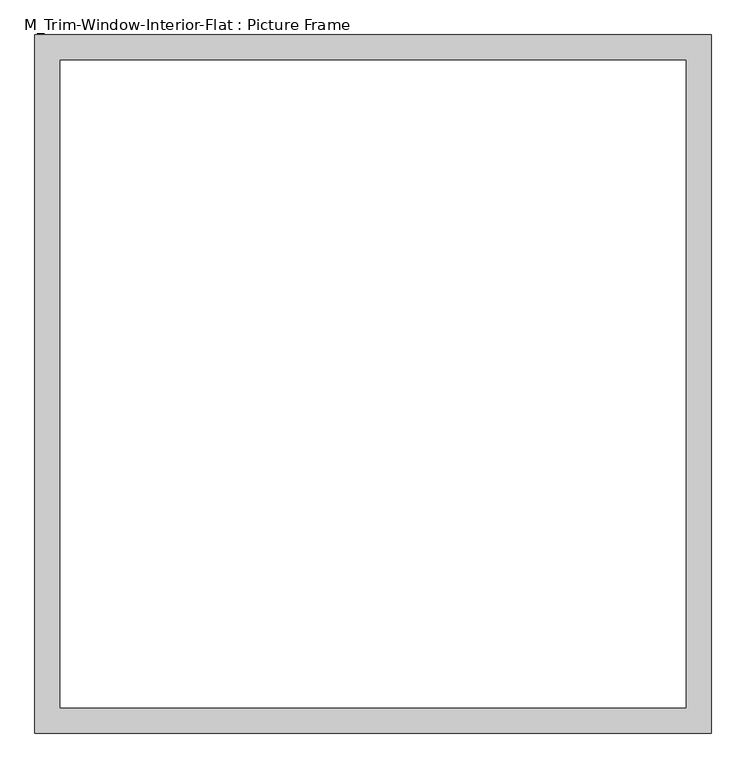
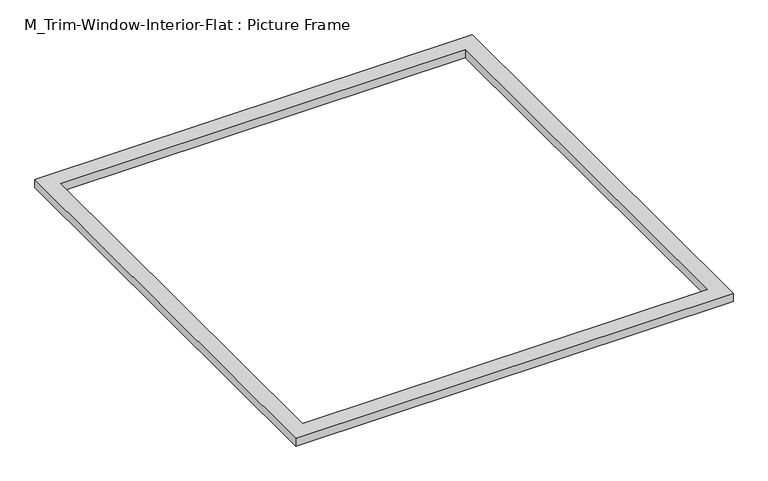
"""IFC4 building model written with IfcOpenShell, lengths in millimetres: proxy geometry, M_Trim-Window-Interior-Flat : Picture Frame."""

from ifc_helpers import new_model, si_unit, origin, origin_with_axes, place, context, project, spatial, polyline, outline, extrude, source, transform, mapped, element, save


def m_trim_window_interior_flat_picture_frame_44e8afef(model_context):
    return source(origin(), model_context, "Body", "SweptSolid", [
        extrude(outline(polyline([(797.3, 47.3), (797.3, -1598.1), (-797.3, -1598.1), (-797.3, 47.3), (797.3, 47.3)]), holes=[polyline([(737.3, -12.7), (-737.3, -12.7), (-737.3, -1538.1), (737.3, -1538.1), (737.3, -12.7)])]), origin_with_axes(), (0.0, 0.0, 1.0), 30.0),
    ])


if __name__ == "__main__":
    model = new_model("IFC4")
    model_context = context("Model", 3, world=origin())
    ifc_project = project(units=[si_unit("LENGTHUNIT", "METRE", prefix="MILLI")], contexts=[model_context])
    site = spatial("IfcSite", under=ifc_project)
    building = spatial("IfcBuilding", under=site)
    placement = place(None, origin())
    m_trim_window_interior_flat_picture_frame_shape = m_trim_window_interior_flat_picture_frame_44e8afef(model_context)
    element("IfcBuildingElementProxy", 1, Name="M_Trim-Window-Interior-Flat : Picture Frame", ObjectType="M_Trim-Window-Interior-Flat : Picture Frame", at=placement, inside=building, context=model_context, shape_type="MappedRepresentation", body=[
        mapped(m_trim_window_interior_flat_picture_frame_shape, transform((0.0, 0.0, 0.0), x_axis=(1.0, 0.0, 0.0), y_axis=(0.0, 1.0, 0.0), z_axis=(0.0, 0.0, 1.0))),
    ])
    save(model, "model.ifc")

# Revit data of these elements
# Type "M_Trim-Window-Interior-Flat : Picture Frame"
#   Trim Thickness_Picture Frame = 0' - 1.1811"
#   Trim Width = 0' - 2.3622"
#   Trim Thickness_with Sill = 0' - 0.7874"
#   Sill Thickness = 0' - 1.1811"
#   Opening Width [instance default] = 1' - 11.62205"
#   Opening Height [instance default] = 2' - 11.43307"
#   Default Elevation = 3' - 11.24409"
#   Sill = no
#   Picture Frame = yes
#   Trim Material [instance default] = none
# Element 1 (IfcBuildingElementProxy, "M_Trim-Window-Interior-Flat : Picture Frame")
#   Opening Width = 4' - 11.05512"
#   Opening Height = 5' - 1.05512"
#   Trim Material = Wood - Stained
#   Materials on its faces: "Wood - Stained"
# Materials
#   "Wood - Stained": class "Wood", colour RGB 224 178 126, transparency 0, Cost = 0
